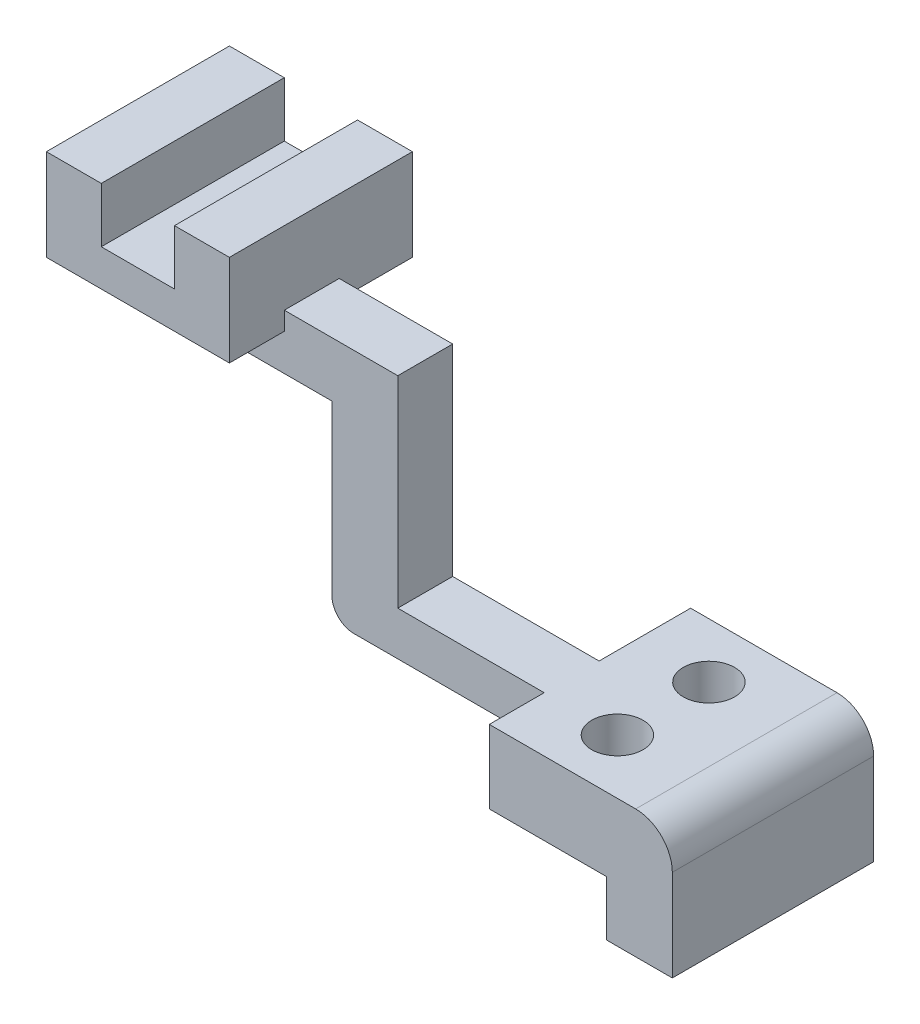
ISO-10303-21;
HEADER;
FILE_DESCRIPTION(('STEP AP214'),'2;1');
FILE_NAME('part.step','',(''),(''),'','','');
FILE_SCHEMA(('AUTOMOTIVE_DESIGN { 1 0 10303 214 1 1 1 1 }'));
ENDSEC;
DATA;
#1=APPLICATION_CONTEXT('core data for automotive mechanical design processes');
#2=APPLICATION_PROTOCOL_DEFINITION('international standard','automotive_design',2000,#1);
#3=PRODUCT_CONTEXT('',#1,'mechanical');
#4=PRODUCT('Part','Part','',(#3));
#5=PRODUCT_RELATED_PRODUCT_CATEGORY('part','',(#4));
#6=PRODUCT_DEFINITION_FORMATION('','',#4);
#7=PRODUCT_DEFINITION_CONTEXT('part definition',#1,'design');
#8=PRODUCT_DEFINITION('design','',#6,#7);
#9=PRODUCT_DEFINITION_SHAPE('','',#8);
#10=(LENGTH_UNIT() NAMED_UNIT(*) SI_UNIT(.MILLI.,.METRE.));
#11=(NAMED_UNIT(*) PLANE_ANGLE_UNIT() SI_UNIT($,.RADIAN.));
#12=(NAMED_UNIT(*) SI_UNIT($,.STERADIAN.) SOLID_ANGLE_UNIT());
#13=UNCERTAINTY_MEASURE_WITH_UNIT(LENGTH_MEASURE(1.E-05),#10,'distance_accuracy_value','');
#14=(GEOMETRIC_REPRESENTATION_CONTEXT(3) GLOBAL_UNCERTAINTY_ASSIGNED_CONTEXT((#13)) GLOBAL_UNIT_ASSIGNED_CONTEXT((#10,
#11,#12)) REPRESENTATION_CONTEXT('',''));
#15=CARTESIAN_POINT('',(0.,0.,0.));
#16=DIRECTION('',(0.,0.,1.));
#17=DIRECTION('',(1.,0.,0.));
#18=AXIS2_PLACEMENT_3D('',#15,#16,#17);
#19=CARTESIAN_POINT('',(-40.,0.,40.));
#20=DIRECTION('',(0.,0.,-1.));
#21=DIRECTION('',(-1.,0.,0.));
#22=AXIS2_PLACEMENT_3D('',#19,#20,#21);
#23=PLANE('',#22);
#24=DIRECTION('',(1.,0.,0.));
#25=VECTOR('',#24,1.);
#26=CARTESIAN_POINT('',(-121.,50.,40.));
#27=LINE('',#26,#25);
#28=CARTESIAN_POINT('',(-121.,50.,40.));
#29=VERTEX_POINT('',#28);
#30=CARTESIAN_POINT('',(-71.,50.,40.));
#31=VERTEX_POINT('',#30);
#32=EDGE_CURVE('E67',#29,#31,#27,.T.);
#33=ORIENTED_EDGE('',*,*,#32,.F.);
#34=DIRECTION('',(0.,-1.,0.));
#35=VECTOR('',#34,1.);
#36=CARTESIAN_POINT('',(-121.,40.,40.));
#37=LINE('',#36,#35);
#38=CARTESIAN_POINT('',(-121.,40.,40.));
#39=VERTEX_POINT('',#38);
#40=EDGE_CURVE('E332',#29,#39,#37,.T.);
#41=ORIENTED_EDGE('',*,*,#40,.T.);
#42=DIRECTION('',(1.,0.,0.));
#43=VECTOR('',#42,1.);
#44=CARTESIAN_POINT('',(-58.,40.,40.));
#45=LINE('',#44,#43);
#46=CARTESIAN_POINT('',(-58.,40.,40.));
#47=VERTEX_POINT('',#46);
#48=EDGE_CURVE('E333',#39,#47,#45,.T.);
#49=ORIENTED_EDGE('',*,*,#48,.T.);
#50=DIRECTION('',(0.,-1.,0.));
#51=VECTOR('',#50,1.);
#52=CARTESIAN_POINT('',(-58.,-6.00000000000004,40.));
#53=LINE('',#52,#51);
#54=CARTESIAN_POINT('',(-58.,-6.00000000000004,40.));
#55=VERTEX_POINT('',#54);
#56=EDGE_CURVE('E340',#47,#55,#53,.T.);
#57=ORIENTED_EDGE('',*,*,#56,.T.);
#58=CARTESIAN_POINT('',(-52.,-6.,40.));
#59=DIRECTION('',(0.,0.,1.));
#60=DIRECTION('',(1.,0.,0.));
#61=AXIS2_PLACEMENT_3D('',#58,#59,#60);
#62=CIRCLE('',#61,6.);
#63=CARTESIAN_POINT('',(-52.,-12.,40.));
#64=VERTEX_POINT('',#63);
#65=EDGE_CURVE('E308',#55,#64,#62,.T.);
#66=ORIENTED_EDGE('',*,*,#65,.T.);
#67=DIRECTION('',(1.,0.,0.));
#68=VECTOR('',#67,1.);
#69=CARTESIAN_POINT('',(-40.,-12.,40.));
#70=LINE('',#69,#68);
#71=CARTESIAN_POINT('',(0.,-12.,40.));
#72=VERTEX_POINT('',#71);
#73=EDGE_CURVE('E373',#64,#72,#70,.T.);
#74=ORIENTED_EDGE('',*,*,#73,.T.);
#75=DIRECTION('',(0.,1.,0.));
#76=VECTOR('',#75,1.);
#77=CARTESIAN_POINT('',(0.,0.,40.));
#78=LINE('',#77,#76);
#79=CARTESIAN_POINT('',(0.,0.,40.));
#80=VERTEX_POINT('',#79);
#81=EDGE_CURVE('E359',#72,#80,#78,.T.);
#82=ORIENTED_EDGE('',*,*,#81,.T.);
#83=DIRECTION('',(1.,0.,0.));
#84=VECTOR('',#83,1.);
#85=CARTESIAN_POINT('',(-40.,0.,40.));
#86=LINE('',#85,#84);
#87=CARTESIAN_POINT('',(-40.,0.,40.));
#88=VERTEX_POINT('',#87);
#89=EDGE_CURVE('E369',#88,#80,#86,.T.);
#90=ORIENTED_EDGE('',*,*,#89,.F.);
#91=DIRECTION('',(0.,1.,0.));
#92=VECTOR('',#91,1.);
#93=CARTESIAN_POINT('',(-40.,55.,40.));
#94=LINE('',#93,#92);
#95=CARTESIAN_POINT('',(-40.,55.,40.));
#96=VERTEX_POINT('',#95);
#97=EDGE_CURVE('E229',#88,#96,#94,.T.);
#98=ORIENTED_EDGE('',*,*,#97,.T.);
#99=DIRECTION('',(-1.,0.,0.));
#100=VECTOR('',#99,1.);
#101=CARTESIAN_POINT('',(-71.,55.,40.));
#102=LINE('',#101,#100);
#103=CARTESIAN_POINT('',(-71.,55.,40.));
#104=VERTEX_POINT('',#103);
#105=EDGE_CURVE('E329',#96,#104,#102,.T.);
#106=ORIENTED_EDGE('',*,*,#105,.T.);
#107=DIRECTION('',(0.,1.,0.));
#108=VECTOR('',#107,1.);
#109=CARTESIAN_POINT('',(-71.,50.,40.));
#110=LINE('',#109,#108);
#111=EDGE_CURVE('E61',#31,#104,#110,.T.);
#112=ORIENTED_EDGE('',*,*,#111,.F.);
#113=EDGE_LOOP('',(#33,#41,#49,#57,#66,#74,#82,#90,#98,#106,#112));
#114=FACE_BOUND('',#113,.T.);
#115=ADVANCED_FACE('F50',(#114),#23,.F.);
#116=CARTESIAN_POINT('',(0.,0.,55.));
#117=DIRECTION('',(1.,0.,0.));
#118=DIRECTION('',(0.,1.,0.));
#119=AXIS2_PLACEMENT_3D('',#116,#117,#118);
#120=PLANE('',#119);
#121=DIRECTION('',(0.,-1.,0.));
#122=VECTOR('',#121,1.);
#123=CARTESIAN_POINT('',(0.,0.,25.));
#124=LINE('',#123,#122);
#125=CARTESIAN_POINT('',(0.,0.,25.));
#126=VERTEX_POINT('',#125);
#127=CARTESIAN_POINT('',(0.,-12.,25.));
#128=VERTEX_POINT('',#127);
#129=EDGE_CURVE('E343',#126,#128,#124,.T.);
#130=ORIENTED_EDGE('',*,*,#129,.F.);
#131=DIRECTION('',(0.,0.,-1.));
#132=VECTOR('',#131,1.);
#133=CARTESIAN_POINT('',(0.,0.,55.));
#134=LINE('',#133,#132);
#135=CARTESIAN_POINT('',(0.,0.,0.));
#136=VERTEX_POINT('',#135);
#137=EDGE_CURVE('E433',#126,#136,#134,.T.);
#138=ORIENTED_EDGE('',*,*,#137,.T.);
#139=DIRECTION('',(0.,-1.,0.));
#140=VECTOR('',#139,1.);
#141=CARTESIAN_POINT('',(0.,0.,0.));
#142=LINE('',#141,#140);
#143=CARTESIAN_POINT('',(0.,-20.,0.));
#144=VERTEX_POINT('',#143);
#145=EDGE_CURVE('E414',#136,#144,#142,.T.);
#146=ORIENTED_EDGE('',*,*,#145,.T.);
#147=DIRECTION('',(0.,0.,-1.));
#148=VECTOR('',#147,1.);
#149=CARTESIAN_POINT('',(0.,-20.,55.));
#150=LINE('',#149,#148);
#151=CARTESIAN_POINT('',(0.,-20.,55.));
#152=VERTEX_POINT('',#151);
#153=EDGE_CURVE('E427',#152,#144,#150,.T.);
#154=ORIENTED_EDGE('',*,*,#153,.F.);
#155=DIRECTION('',(0.,-1.,0.));
#156=VECTOR('',#155,1.);
#157=CARTESIAN_POINT('',(0.,0.,55.));
#158=LINE('',#157,#156);
#159=CARTESIAN_POINT('',(0.,0.,55.));
#160=VERTEX_POINT('',#159);
#161=EDGE_CURVE('E394',#160,#152,#158,.T.);
#162=ORIENTED_EDGE('',*,*,#161,.F.);
#163=EDGE_CURVE('E432',#160,#80,#134,.T.);
#164=ORIENTED_EDGE('',*,*,#163,.T.);
#165=ORIENTED_EDGE('',*,*,#81,.F.);
#166=DIRECTION('',(0.,0.,1.));
#167=VECTOR('',#166,1.);
#168=CARTESIAN_POINT('',(0.,-12.,25.));
#169=LINE('',#168,#167);
#170=EDGE_CURVE('E361',#128,#72,#169,.T.);
#171=ORIENTED_EDGE('',*,*,#170,.F.);
#172=EDGE_LOOP('',(#130,#138,#146,#154,#162,#164,#165,#171));
#173=FACE_BOUND('',#172,.T.);
#174=ADVANCED_FACE('F462',(#173),#120,.F.);
#175=CARTESIAN_POINT('',(50.,0.,55.));
#176=DIRECTION('',(1.,0.,0.));
#177=DIRECTION('',(0.,0.,-1.));
#178=AXIS2_PLACEMENT_3D('',#175,#176,#177);
#179=PLANE('',#178);
#180=DIRECTION('',(0.,-1.,0.));
#181=VECTOR('',#180,1.);
#182=CARTESIAN_POINT('',(50.,0.,0.));
#183=LINE('',#182,#181);
#184=CARTESIAN_POINT('',(50.,-10.,0.));
#185=VERTEX_POINT('',#184);
#186=CARTESIAN_POINT('',(50.,-35.,0.));
#187=VERTEX_POINT('',#186);
#188=EDGE_CURVE('E407',#185,#187,#183,.T.);
#189=ORIENTED_EDGE('',*,*,#188,.F.);
#190=DIRECTION('',(0.,0.,-1.));
#191=VECTOR('',#190,1.);
#192=CARTESIAN_POINT('',(50.,-10.,55.));
#193=LINE('',#192,#191);
#194=CARTESIAN_POINT('',(50.,-10.,55.));
#195=VERTEX_POINT('',#194);
#196=EDGE_CURVE('E11',#195,#185,#193,.T.);
#197=ORIENTED_EDGE('',*,*,#196,.F.);
#198=DIRECTION('',(0.,-1.,0.));
#199=VECTOR('',#198,1.);
#200=CARTESIAN_POINT('',(50.,0.,55.));
#201=LINE('',#200,#199);
#202=CARTESIAN_POINT('',(50.,-35.,55.));
#203=VERTEX_POINT('',#202);
#204=EDGE_CURVE('E387',#195,#203,#201,.T.);
#205=ORIENTED_EDGE('',*,*,#204,.T.);
#206=DIRECTION('',(0.,0.,-1.));
#207=VECTOR('',#206,1.);
#208=CARTESIAN_POINT('',(50.,-35.,55.));
#209=LINE('',#208,#207);
#210=EDGE_CURVE('E403',#203,#187,#209,.T.);
#211=ORIENTED_EDGE('',*,*,#210,.T.);
#212=EDGE_LOOP('',(#189,#197,#205,#211));
#213=FACE_BOUND('',#212,.T.);
#214=ADVANCED_FACE('F47',(#213),#179,.T.);
#215=CARTESIAN_POINT('',(40.,-10.,55.));
#216=DIRECTION('',(0.,0.,-1.));
#217=DIRECTION('',(-1.,0.,0.));
#218=AXIS2_PLACEMENT_3D('',#215,#216,#217);
#219=CYLINDRICAL_SURFACE('',#218,10.);
#220=CARTESIAN_POINT('',(40.,-10.,0.));
#221=DIRECTION('',(0.,0.,1.));
#222=DIRECTION('',(1.,0.,0.));
#223=AXIS2_PLACEMENT_3D('',#220,#221,#222);
#224=CIRCLE('',#223,10.);
#225=CARTESIAN_POINT('',(40.,0.,0.));
#226=VERTEX_POINT('',#225);
#227=EDGE_CURVE('E406',#185,#226,#224,.T.);
#228=ORIENTED_EDGE('',*,*,#227,.T.);
#229=DIRECTION('',(0.,0.,-1.));
#230=VECTOR('',#229,1.);
#231=CARTESIAN_POINT('',(40.,0.,55.));
#232=LINE('',#231,#230);
#233=CARTESIAN_POINT('',(40.,0.,55.));
#234=VERTEX_POINT('',#233);
#235=EDGE_CURVE('E57',#234,#226,#232,.T.);
#236=ORIENTED_EDGE('',*,*,#235,.F.);
#237=CARTESIAN_POINT('',(40.,-10.,55.));
#238=DIRECTION('',(0.,0.,1.));
#239=DIRECTION('',(1.,0.,0.));
#240=AXIS2_PLACEMENT_3D('',#237,#238,#239);
#241=CIRCLE('',#240,10.);
#242=EDGE_CURVE('E386',#195,#234,#241,.T.);
#243=ORIENTED_EDGE('',*,*,#242,.F.);
#244=ORIENTED_EDGE('',*,*,#196,.T.);
#245=EDGE_LOOP('',(#228,#236,#243,#244));
#246=FACE_BOUND('',#245,.T.);
#247=ADVANCED_FACE('F827',(#246),#219,.T.);
#248=CARTESIAN_POINT('',(0.,0.,55.));
#249=DIRECTION('',(0.,1.,0.));
#250=DIRECTION('',(0.,0.,1.));
#251=AXIS2_PLACEMENT_3D('',#248,#249,#250);
#252=PLANE('',#251);
#253=ORIENTED_EDGE('',*,*,#137,.F.);
#254=DIRECTION('',(1.,0.,0.));
#255=VECTOR('',#254,1.);
#256=CARTESIAN_POINT('',(-40.,0.,25.));
#257=LINE('',#256,#255);
#258=CARTESIAN_POINT('',(-40.,0.,25.));
#259=VERTEX_POINT('',#258);
#260=EDGE_CURVE('E360',#259,#126,#257,.T.);
#261=ORIENTED_EDGE('',*,*,#260,.F.);
#262=DIRECTION('',(0.,0.,-1.));
#263=VECTOR('',#262,1.);
#264=CARTESIAN_POINT('',(-40.,0.,25.));
#265=LINE('',#264,#263);
#266=EDGE_CURVE('E358',#88,#259,#265,.T.);
#267=ORIENTED_EDGE('',*,*,#266,.F.);
#268=ORIENTED_EDGE('',*,*,#89,.T.);
#269=ORIENTED_EDGE('',*,*,#163,.F.);
#270=DIRECTION('',(1.,0.,0.));
#271=VECTOR('',#270,1.);
#272=CARTESIAN_POINT('',(0.,0.,55.));
#273=LINE('',#272,#271);
#274=EDGE_CURVE('E395',#160,#234,#273,.T.);
#275=ORIENTED_EDGE('',*,*,#274,.T.);
#276=ORIENTED_EDGE('',*,*,#235,.T.);
#277=DIRECTION('',(1.,0.,0.));
#278=VECTOR('',#277,1.);
#279=CARTESIAN_POINT('',(0.,0.,0.));
#280=LINE('',#279,#278);
#281=EDGE_CURVE('E415',#136,#226,#280,.T.);
#282=ORIENTED_EDGE('',*,*,#281,.F.);
#283=EDGE_LOOP('',(#253,#261,#267,#268,#269,#275,#276,#282));
#284=FACE_BOUND('',#283,.T.);
#285=CARTESIAN_POINT('',(20.,0.,15.));
#286=DIRECTION('',(0.,1.,0.));
#287=DIRECTION('',(0.,0.,1.));
#288=AXIS2_PLACEMENT_3D('',#285,#286,#287);
#289=CIRCLE('',#288,7.);
#290=CARTESIAN_POINT('',(20.,0.,22.));
#291=VERTEX_POINT('',#290);
#292=EDGE_CURVE('E379',#291,#291,#289,.T.);
#293=ORIENTED_EDGE('',*,*,#292,.F.);
#294=EDGE_LOOP('',(#293));
#295=FACE_BOUND('',#294,.T.);
#296=CARTESIAN_POINT('',(20.,0.,40.));
#297=DIRECTION('',(0.,1.,0.));
#298=DIRECTION('',(0.,0.,1.));
#299=AXIS2_PLACEMENT_3D('',#296,#297,#298);
#300=CIRCLE('',#299,7.);
#301=CARTESIAN_POINT('',(20.,0.,47.));
#302=VERTEX_POINT('',#301);
#303=EDGE_CURVE('E378',#302,#302,#300,.T.);
#304=ORIENTED_EDGE('',*,*,#303,.F.);
#305=EDGE_LOOP('',(#304));
#306=FACE_BOUND('',#305,.T.);
#307=ADVANCED_FACE('F516',(#284,#295,#306),#252,.T.);
#308=CARTESIAN_POINT('',(0.,-20.,55.));
#309=DIRECTION('',(0.,1.,0.));
#310=DIRECTION('',(0.,0.,1.));
#311=AXIS2_PLACEMENT_3D('',#308,#309,#310);
#312=PLANE('',#311);
#313=CARTESIAN_POINT('',(20.,-20.,15.));
#314=DIRECTION('',(0.,1.,0.));
#315=DIRECTION('',(0.,0.,1.));
#316=AXIS2_PLACEMENT_3D('',#313,#314,#315);
#317=CIRCLE('',#316,7.);
#318=CARTESIAN_POINT('',(20.,-20.,22.));
#319=VERTEX_POINT('',#318);
#320=EDGE_CURVE('E51',#319,#319,#317,.T.);
#321=ORIENTED_EDGE('',*,*,#320,.T.);
#322=EDGE_LOOP('',(#321));
#323=FACE_BOUND('',#322,.T.);
#324=CARTESIAN_POINT('',(20.,-20.,40.));
#325=DIRECTION('',(0.,1.,0.));
#326=DIRECTION('',(0.,0.,1.));
#327=AXIS2_PLACEMENT_3D('',#324,#325,#326);
#328=CIRCLE('',#327,7.);
#329=CARTESIAN_POINT('',(20.,-20.,47.));
#330=VERTEX_POINT('',#329);
#331=EDGE_CURVE('E384',#330,#330,#328,.T.);
#332=ORIENTED_EDGE('',*,*,#331,.T.);
#333=EDGE_LOOP('',(#332));
#334=FACE_BOUND('',#333,.T.);
#335=DIRECTION('',(1.,0.,0.));
#336=VECTOR('',#335,1.);
#337=CARTESIAN_POINT('',(0.,-20.,0.));
#338=LINE('',#337,#336);
#339=CARTESIAN_POINT('',(32.,-20.,0.));
#340=VERTEX_POINT('',#339);
#341=EDGE_CURVE('E417',#144,#340,#338,.T.);
#342=ORIENTED_EDGE('',*,*,#341,.T.);
#343=DIRECTION('',(0.,0.,-1.));
#344=VECTOR('',#343,1.);
#345=CARTESIAN_POINT('',(32.,-20.,55.));
#346=LINE('',#345,#344);
#347=CARTESIAN_POINT('',(32.,-20.,55.));
#348=VERTEX_POINT('',#347);
#349=EDGE_CURVE('E426',#348,#340,#346,.T.);
#350=ORIENTED_EDGE('',*,*,#349,.F.);
#351=DIRECTION('',(1.,0.,0.));
#352=VECTOR('',#351,1.);
#353=CARTESIAN_POINT('',(0.,-20.,55.));
#354=LINE('',#353,#352);
#355=EDGE_CURVE('E397',#152,#348,#354,.T.);
#356=ORIENTED_EDGE('',*,*,#355,.F.);
#357=ORIENTED_EDGE('',*,*,#153,.T.);
#358=EDGE_LOOP('',(#342,#350,#356,#357));
#359=FACE_BOUND('',#358,.T.);
#360=ADVANCED_FACE('F445',(#323,#334,#359),#312,.F.);
#361=CARTESIAN_POINT('',(32.,0.,55.));
#362=DIRECTION('',(-1.,0.,0.));
#363=DIRECTION('',(0.,0.,1.));
#364=AXIS2_PLACEMENT_3D('',#361,#362,#363);
#365=PLANE('',#364);
#366=DIRECTION('',(0.,1.,0.));
#367=VECTOR('',#366,1.);
#368=CARTESIAN_POINT('',(32.,0.,0.));
#369=LINE('',#368,#367);
#370=CARTESIAN_POINT('',(32.,-35.,0.));
#371=VERTEX_POINT('',#370);
#372=EDGE_CURVE('E420',#371,#340,#369,.T.);
#373=ORIENTED_EDGE('',*,*,#372,.F.);
#374=DIRECTION('',(0.,0.,-1.));
#375=VECTOR('',#374,1.);
#376=CARTESIAN_POINT('',(32.,-35.,55.));
#377=LINE('',#376,#375);
#378=CARTESIAN_POINT('',(32.,-35.,55.));
#379=VERTEX_POINT('',#378);
#380=EDGE_CURVE('E428',#379,#371,#377,.T.);
#381=ORIENTED_EDGE('',*,*,#380,.F.);
#382=DIRECTION('',(0.,1.,0.));
#383=VECTOR('',#382,1.);
#384=CARTESIAN_POINT('',(32.,0.,55.));
#385=LINE('',#384,#383);
#386=EDGE_CURVE('E398',#379,#348,#385,.T.);
#387=ORIENTED_EDGE('',*,*,#386,.T.);
#388=ORIENTED_EDGE('',*,*,#349,.T.);
#389=EDGE_LOOP('',(#373,#381,#387,#388));
#390=FACE_BOUND('',#389,.T.);
#391=ADVANCED_FACE('F804',(#390),#365,.T.);
#392=CARTESIAN_POINT('',(0.,-35.,55.));
#393=DIRECTION('',(0.,-1.,0.));
#394=DIRECTION('',(0.,0.,-1.));
#395=AXIS2_PLACEMENT_3D('',#392,#393,#394);
#396=PLANE('',#395);
#397=DIRECTION('',(-1.,0.,0.));
#398=VECTOR('',#397,1.);
#399=CARTESIAN_POINT('',(0.,-35.,0.));
#400=LINE('',#399,#398);
#401=EDGE_CURVE('E388',#187,#371,#400,.T.);
#402=ORIENTED_EDGE('',*,*,#401,.F.);
#403=ORIENTED_EDGE('',*,*,#210,.F.);
#404=DIRECTION('',(-1.,0.,0.));
#405=VECTOR('',#404,1.);
#406=CARTESIAN_POINT('',(0.,-35.,55.));
#407=LINE('',#406,#405);
#408=EDGE_CURVE('E405',#203,#379,#407,.T.);
#409=ORIENTED_EDGE('',*,*,#408,.T.);
#410=ORIENTED_EDGE('',*,*,#380,.T.);
#411=EDGE_LOOP('',(#402,#403,#409,#410));
#412=FACE_BOUND('',#411,.T.);
#413=ADVANCED_FACE('F800',(#412),#396,.T.);
#414=CARTESIAN_POINT('',(0.,0.,55.));
#415=DIRECTION('',(0.,0.,1.));
#416=DIRECTION('',(1.,0.,0.));
#417=AXIS2_PLACEMENT_3D('',#414,#415,#416);
#418=PLANE('',#417);
#419=ORIENTED_EDGE('',*,*,#204,.F.);
#420=ORIENTED_EDGE('',*,*,#242,.T.);
#421=ORIENTED_EDGE('',*,*,#274,.F.);
#422=ORIENTED_EDGE('',*,*,#161,.T.);
#423=ORIENTED_EDGE('',*,*,#355,.T.);
#424=ORIENTED_EDGE('',*,*,#386,.F.);
#425=ORIENTED_EDGE('',*,*,#408,.F.);
#426=EDGE_LOOP('',(#419,#420,#421,#422,#423,#424,#425));
#427=FACE_BOUND('',#426,.T.);
#428=ADVANCED_FACE('F533',(#427),#418,.T.);
#429=CARTESIAN_POINT('',(0.,0.,0.));
#430=DIRECTION('',(0.,0.,1.));
#431=DIRECTION('',(1.,0.,0.));
#432=AXIS2_PLACEMENT_3D('',#429,#430,#431);
#433=PLANE('',#432);
#434=ORIENTED_EDGE('',*,*,#188,.T.);
#435=ORIENTED_EDGE('',*,*,#401,.T.);
#436=ORIENTED_EDGE('',*,*,#372,.T.);
#437=ORIENTED_EDGE('',*,*,#341,.F.);
#438=ORIENTED_EDGE('',*,*,#145,.F.);
#439=ORIENTED_EDGE('',*,*,#281,.T.);
#440=ORIENTED_EDGE('',*,*,#227,.F.);
#441=EDGE_LOOP('',(#434,#435,#436,#437,#438,#439,#440));
#442=FACE_BOUND('',#441,.T.);
#443=ADVANCED_FACE('F457',(#442),#433,.F.);
#444=CARTESIAN_POINT('',(20.,-22.,40.));
#445=DIRECTION('',(0.,1.,0.));
#446=DIRECTION('',(0.,0.,1.));
#447=AXIS2_PLACEMENT_3D('',#444,#445,#446);
#448=CYLINDRICAL_SURFACE('',#447,7.);
#449=ORIENTED_EDGE('',*,*,#303,.T.);
#450=EDGE_LOOP('',(#449));
#451=FACE_BOUND('',#450,.T.);
#452=ORIENTED_EDGE('',*,*,#331,.F.);
#453=EDGE_LOOP('',(#452));
#454=FACE_BOUND('',#453,.T.);
#455=ADVANCED_FACE('F450',(#451,#454),#448,.F.);
#456=CARTESIAN_POINT('',(20.,-22.,15.));
#457=DIRECTION('',(0.,1.,0.));
#458=DIRECTION('',(0.,0.,1.));
#459=AXIS2_PLACEMENT_3D('',#456,#457,#458);
#460=CYLINDRICAL_SURFACE('',#459,7.);
#461=ORIENTED_EDGE('',*,*,#292,.T.);
#462=EDGE_LOOP('',(#461));
#463=FACE_BOUND('',#462,.T.);
#464=ORIENTED_EDGE('',*,*,#320,.F.);
#465=EDGE_LOOP('',(#464));
#466=FACE_BOUND('',#465,.T.);
#467=ADVANCED_FACE('F443',(#463,#466),#460,.F.);
#468=CARTESIAN_POINT('',(-40.,0.,25.));
#469=DIRECTION('',(0.,0.,1.));
#470=DIRECTION('',(1.,0.,0.));
#471=AXIS2_PLACEMENT_3D('',#468,#469,#470);
#472=PLANE('',#471);
#473=ORIENTED_EDGE('',*,*,#129,.T.);
#474=DIRECTION('',(1.,0.,0.));
#475=VECTOR('',#474,1.);
#476=CARTESIAN_POINT('',(-40.,-12.,25.));
#477=LINE('',#476,#475);
#478=CARTESIAN_POINT('',(-52.,-12.,25.));
#479=VERTEX_POINT('',#478);
#480=EDGE_CURVE('E376',#479,#128,#477,.T.);
#481=ORIENTED_EDGE('',*,*,#480,.F.);
#482=CARTESIAN_POINT('',(-52.,-6.,25.));
#483=DIRECTION('',(0.,0.,1.));
#484=DIRECTION('',(1.,0.,0.));
#485=AXIS2_PLACEMENT_3D('',#482,#483,#484);
#486=CIRCLE('',#485,6.);
#487=CARTESIAN_POINT('',(-58.,-6.00000000000004,25.));
#488=VERTEX_POINT('',#487);
#489=EDGE_CURVE('E321',#488,#479,#486,.T.);
#490=ORIENTED_EDGE('',*,*,#489,.F.);
#491=DIRECTION('',(0.,-1.,0.));
#492=VECTOR('',#491,1.);
#493=CARTESIAN_POINT('',(-58.,-6.00000000000004,25.));
#494=LINE('',#493,#492);
#495=CARTESIAN_POINT('',(-58.,40.,25.));
#496=VERTEX_POINT('',#495);
#497=EDGE_CURVE('E322',#496,#488,#494,.T.);
#498=ORIENTED_EDGE('',*,*,#497,.F.);
#499=DIRECTION('',(1.,0.,0.));
#500=VECTOR('',#499,1.);
#501=CARTESIAN_POINT('',(-58.,40.,25.));
#502=LINE('',#501,#500);
#503=CARTESIAN_POINT('',(-121.,40.,25.));
#504=VERTEX_POINT('',#503);
#505=EDGE_CURVE('E319',#504,#496,#502,.T.);
#506=ORIENTED_EDGE('',*,*,#505,.F.);
#507=DIRECTION('',(0.,-1.,0.));
#508=VECTOR('',#507,1.);
#509=CARTESIAN_POINT('',(-121.,40.,25.));
#510=LINE('',#509,#508);
#511=CARTESIAN_POINT('',(-121.,50.,25.));
#512=VERTEX_POINT('',#511);
#513=EDGE_CURVE('E314',#512,#504,#510,.T.);
#514=ORIENTED_EDGE('',*,*,#513,.F.);
#515=DIRECTION('',(-1.,0.,0.));
#516=VECTOR('',#515,1.);
#517=CARTESIAN_POINT('',(-121.,50.,25.));
#518=LINE('',#517,#516);
#519=CARTESIAN_POINT('',(-71.,50.,25.));
#520=VERTEX_POINT('',#519);
#521=EDGE_CURVE('E312',#520,#512,#518,.T.);
#522=ORIENTED_EDGE('',*,*,#521,.F.);
#523=DIRECTION('',(0.,-1.,0.));
#524=VECTOR('',#523,1.);
#525=CARTESIAN_POINT('',(-71.,50.,25.));
#526=LINE('',#525,#524);
#527=CARTESIAN_POINT('',(-71.,55.,25.));
#528=VERTEX_POINT('',#527);
#529=EDGE_CURVE('E311',#528,#520,#526,.T.);
#530=ORIENTED_EDGE('',*,*,#529,.F.);
#531=DIRECTION('',(-1.,0.,0.));
#532=VECTOR('',#531,1.);
#533=CARTESIAN_POINT('',(-71.,55.,25.));
#534=LINE('',#533,#532);
#535=CARTESIAN_POINT('',(-40.,55.,25.));
#536=VERTEX_POINT('',#535);
#537=EDGE_CURVE('E310',#536,#528,#534,.T.);
#538=ORIENTED_EDGE('',*,*,#537,.F.);
#539=DIRECTION('',(0.,1.,0.));
#540=VECTOR('',#539,1.);
#541=CARTESIAN_POINT('',(-40.,55.,25.));
#542=LINE('',#541,#540);
#543=EDGE_CURVE('E302',#259,#536,#542,.T.);
#544=ORIENTED_EDGE('',*,*,#543,.F.);
#545=ORIENTED_EDGE('',*,*,#260,.T.);
#546=EDGE_LOOP('',(#473,#481,#490,#498,#506,#514,#522,#530,#538,#544,#545));
#547=FACE_BOUND('',#546,.T.);
#548=ADVANCED_FACE('F447',(#547),#472,.F.);
#549=CARTESIAN_POINT('',(-40.,-12.,25.));
#550=DIRECTION('',(0.,1.,0.));
#551=DIRECTION('',(-1.,0.,0.));
#552=AXIS2_PLACEMENT_3D('',#549,#550,#551);
#553=PLANE('',#552);
#554=ORIENTED_EDGE('',*,*,#170,.T.);
#555=ORIENTED_EDGE('',*,*,#73,.F.);
#556=DIRECTION('',(0.,0.,1.));
#557=VECTOR('',#556,1.);
#558=CARTESIAN_POINT('',(-52.,-12.,25.));
#559=LINE('',#558,#557);
#560=EDGE_CURVE('E345',#479,#64,#559,.T.);
#561=ORIENTED_EDGE('',*,*,#560,.F.);
#562=ORIENTED_EDGE('',*,*,#480,.T.);
#563=EDGE_LOOP('',(#554,#555,#561,#562));
#564=FACE_BOUND('',#563,.T.);
#565=ADVANCED_FACE('F453',(#564),#553,.F.);
#566=CARTESIAN_POINT('',(-52.,-6.,25.));
#567=DIRECTION('',(0.,0.,1.));
#568=DIRECTION('',(1.,0.,0.));
#569=AXIS2_PLACEMENT_3D('',#566,#567,#568);
#570=CYLINDRICAL_SURFACE('',#569,6.);
#571=ORIENTED_EDGE('',*,*,#65,.F.);
#572=DIRECTION('',(0.,0.,1.));
#573=VECTOR('',#572,1.);
#574=CARTESIAN_POINT('',(-58.,-6.00000000000004,25.));
#575=LINE('',#574,#573);
#576=EDGE_CURVE('E346',#488,#55,#575,.T.);
#577=ORIENTED_EDGE('',*,*,#576,.F.);
#578=ORIENTED_EDGE('',*,*,#489,.T.);
#579=ORIENTED_EDGE('',*,*,#560,.T.);
#580=EDGE_LOOP('',(#571,#577,#578,#579));
#581=FACE_BOUND('',#580,.T.);
#582=ADVANCED_FACE('F476',(#581),#570,.T.);
#583=CARTESIAN_POINT('',(-58.,-6.00000000000004,25.));
#584=DIRECTION('',(-1.,0.,0.));
#585=DIRECTION('',(0.,0.,1.));
#586=AXIS2_PLACEMENT_3D('',#583,#584,#585);
#587=PLANE('',#586);
#588=ORIENTED_EDGE('',*,*,#56,.F.);
#589=DIRECTION('',(0.,0.,1.));
#590=VECTOR('',#589,1.);
#591=CARTESIAN_POINT('',(-58.,40.,25.));
#592=LINE('',#591,#590);
#593=EDGE_CURVE('E347',#496,#47,#592,.T.);
#594=ORIENTED_EDGE('',*,*,#593,.F.);
#595=ORIENTED_EDGE('',*,*,#497,.T.);
#596=ORIENTED_EDGE('',*,*,#576,.T.);
#597=EDGE_LOOP('',(#588,#594,#595,#596));
#598=FACE_BOUND('',#597,.T.);
#599=ADVANCED_FACE('F482',(#598),#587,.T.);
#600=CARTESIAN_POINT('',(-58.,40.,25.));
#601=DIRECTION('',(0.,-1.,0.));
#602=DIRECTION('',(0.,0.,-1.));
#603=AXIS2_PLACEMENT_3D('',#600,#601,#602);
#604=PLANE('',#603);
#605=ORIENTED_EDGE('',*,*,#48,.F.);
#606=DIRECTION('',(0.,0.,1.));
#607=VECTOR('',#606,1.);
#608=CARTESIAN_POINT('',(-121.,40.,25.));
#609=LINE('',#608,#607);
#610=EDGE_CURVE('E349',#504,#39,#609,.T.);
#611=ORIENTED_EDGE('',*,*,#610,.F.);
#612=ORIENTED_EDGE('',*,*,#505,.T.);
#613=ORIENTED_EDGE('',*,*,#593,.T.);
#614=EDGE_LOOP('',(#605,#611,#612,#613));
#615=FACE_BOUND('',#614,.T.);
#616=ADVANCED_FACE('F492',(#615),#604,.T.);
#617=CARTESIAN_POINT('',(-121.,40.,25.));
#618=DIRECTION('',(-1.,0.,0.));
#619=DIRECTION('',(0.,0.,1.));
#620=AXIS2_PLACEMENT_3D('',#617,#618,#619);
#621=PLANE('',#620);
#622=ORIENTED_EDGE('',*,*,#40,.F.);
#623=DIRECTION('',(0.,0.,-1.));
#624=VECTOR('',#623,1.);
#625=CARTESIAN_POINT('',(-121.,50.,55.));
#626=LINE('',#625,#624);
#627=CARTESIAN_POINT('',(-121.,50.,55.));
#628=VERTEX_POINT('',#627);
#629=EDGE_CURVE('E240',#628,#29,#626,.T.);
#630=ORIENTED_EDGE('',*,*,#629,.F.);
#631=DIRECTION('',(0.,-1.,0.));
#632=VECTOR('',#631,1.);
#633=CARTESIAN_POINT('',(-121.,75.,55.));
#634=LINE('',#633,#632);
#635=CARTESIAN_POINT('',(-121.,75.,55.));
#636=VERTEX_POINT('',#635);
#637=EDGE_CURVE('E234',#636,#628,#634,.T.);
#638=ORIENTED_EDGE('',*,*,#637,.F.);
#639=DIRECTION('',(0.,0.,1.));
#640=VECTOR('',#639,1.);
#641=CARTESIAN_POINT('',(-121.,75.,5.));
#642=LINE('',#641,#640);
#643=CARTESIAN_POINT('',(-121.,75.,5.));
#644=VERTEX_POINT('',#643);
#645=EDGE_CURVE('E219',#644,#636,#642,.T.);
#646=ORIENTED_EDGE('',*,*,#645,.F.);
#647=DIRECTION('',(0.,-1.,0.));
#648=VECTOR('',#647,1.);
#649=CARTESIAN_POINT('',(-121.,75.,5.));
#650=LINE('',#649,#648);
#651=CARTESIAN_POINT('',(-121.,50.,5.));
#652=VERTEX_POINT('',#651);
#653=EDGE_CURVE('E269',#644,#652,#650,.T.);
#654=ORIENTED_EDGE('',*,*,#653,.T.);
#655=DIRECTION('',(0.,0.,1.));
#656=VECTOR('',#655,1.);
#657=CARTESIAN_POINT('',(-121.,50.,5.));
#658=LINE('',#657,#656);
#659=EDGE_CURVE('E289',#652,#512,#658,.T.);
#660=ORIENTED_EDGE('',*,*,#659,.T.);
#661=ORIENTED_EDGE('',*,*,#513,.T.);
#662=ORIENTED_EDGE('',*,*,#610,.T.);
#663=EDGE_LOOP('',(#622,#630,#638,#646,#654,#660,#661,#662));
#664=FACE_BOUND('',#663,.T.);
#665=ADVANCED_FACE('F232',(#664),#621,.T.);
#666=CARTESIAN_POINT('',(-71.,55.,25.));
#667=DIRECTION('',(0.,1.,0.));
#668=DIRECTION('',(0.,0.,1.));
#669=AXIS2_PLACEMENT_3D('',#666,#667,#668);
#670=PLANE('',#669);
#671=ORIENTED_EDGE('',*,*,#105,.F.);
#672=DIRECTION('',(0.,0.,1.));
#673=VECTOR('',#672,1.);
#674=CARTESIAN_POINT('',(-40.,55.,25.));
#675=LINE('',#674,#673);
#676=EDGE_CURVE('E330',#536,#96,#675,.T.);
#677=ORIENTED_EDGE('',*,*,#676,.F.);
#678=ORIENTED_EDGE('',*,*,#537,.T.);
#679=DIRECTION('',(0.,0.,1.));
#680=VECTOR('',#679,1.);
#681=CARTESIAN_POINT('',(-71.,55.,25.));
#682=LINE('',#681,#680);
#683=EDGE_CURVE('E354',#528,#104,#682,.T.);
#684=ORIENTED_EDGE('',*,*,#683,.T.);
#685=EDGE_LOOP('',(#671,#677,#678,#684));
#686=FACE_BOUND('',#685,.T.);
#687=ADVANCED_FACE('F511',(#686),#670,.T.);
#688=CARTESIAN_POINT('',(-40.,55.,25.));
#689=DIRECTION('',(1.,0.,0.));
#690=DIRECTION('',(0.,0.,-1.));
#691=AXIS2_PLACEMENT_3D('',#688,#689,#690);
#692=PLANE('',#691);
#693=ORIENTED_EDGE('',*,*,#97,.F.);
#694=ORIENTED_EDGE('',*,*,#266,.T.);
#695=ORIENTED_EDGE('',*,*,#543,.T.);
#696=ORIENTED_EDGE('',*,*,#676,.T.);
#697=EDGE_LOOP('',(#693,#694,#695,#696));
#698=FACE_BOUND('',#697,.T.);
#699=ADVANCED_FACE('F474',(#698),#692,.T.);
#700=CARTESIAN_POINT('',(-121.,50.,5.));
#701=DIRECTION('',(0.,-1.,0.));
#702=DIRECTION('',(0.,0.,-1.));
#703=AXIS2_PLACEMENT_3D('',#700,#701,#702);
#704=PLANE('',#703);
#705=ORIENTED_EDGE('',*,*,#521,.T.);
#706=ORIENTED_EDGE('',*,*,#659,.F.);
#707=DIRECTION('',(1.,0.,0.));
#708=VECTOR('',#707,1.);
#709=CARTESIAN_POINT('',(-121.,50.,5.));
#710=LINE('',#709,#708);
#711=CARTESIAN_POINT('',(-71.,50.,5.));
#712=VERTEX_POINT('',#711);
#713=EDGE_CURVE('E270',#652,#712,#710,.T.);
#714=ORIENTED_EDGE('',*,*,#713,.T.);
#715=DIRECTION('',(0.,0.,1.));
#716=VECTOR('',#715,1.);
#717=CARTESIAN_POINT('',(-71.,50.,5.));
#718=LINE('',#717,#716);
#719=EDGE_CURVE('E299',#712,#520,#718,.T.);
#720=ORIENTED_EDGE('',*,*,#719,.T.);
#721=EDGE_LOOP('',(#705,#706,#714,#720));
#722=FACE_BOUND('',#721,.T.);
#723=ADVANCED_FACE('F499',(#722),#704,.T.);
#724=CARTESIAN_POINT('',(-71.,50.,5.));
#725=DIRECTION('',(1.,0.,0.));
#726=DIRECTION('',(0.,0.,-1.));
#727=AXIS2_PLACEMENT_3D('',#724,#725,#726);
#728=PLANE('',#727);
#729=ORIENTED_EDGE('',*,*,#529,.T.);
#730=ORIENTED_EDGE('',*,*,#719,.F.);
#731=DIRECTION('',(0.,1.,0.));
#732=VECTOR('',#731,1.);
#733=CARTESIAN_POINT('',(-71.,50.,5.));
#734=LINE('',#733,#732);
#735=CARTESIAN_POINT('',(-71.,75.,5.));
#736=VERTEX_POINT('',#735);
#737=EDGE_CURVE('E271',#712,#736,#734,.T.);
#738=ORIENTED_EDGE('',*,*,#737,.T.);
#739=DIRECTION('',(0.,0.,1.));
#740=VECTOR('',#739,1.);
#741=CARTESIAN_POINT('',(-71.,75.,5.));
#742=LINE('',#741,#740);
#743=CARTESIAN_POINT('',(-71.,75.,55.));
#744=VERTEX_POINT('',#743);
#745=EDGE_CURVE('E300',#736,#744,#742,.T.);
#746=ORIENTED_EDGE('',*,*,#745,.T.);
#747=DIRECTION('',(0.,1.,0.));
#748=VECTOR('',#747,1.);
#749=CARTESIAN_POINT('',(-71.,50.,55.));
#750=LINE('',#749,#748);
#751=CARTESIAN_POINT('',(-71.,50.,55.));
#752=VERTEX_POINT('',#751);
#753=EDGE_CURVE('E252',#752,#744,#750,.T.);
#754=ORIENTED_EDGE('',*,*,#753,.F.);
#755=DIRECTION('',(0.,0.,-1.));
#756=VECTOR('',#755,1.);
#757=CARTESIAN_POINT('',(-71.,50.,55.));
#758=LINE('',#757,#756);
#759=EDGE_CURVE('E262',#752,#31,#758,.T.);
#760=ORIENTED_EDGE('',*,*,#759,.T.);
#761=ORIENTED_EDGE('',*,*,#111,.T.);
#762=ORIENTED_EDGE('',*,*,#683,.F.);
#763=EDGE_LOOP('',(#729,#730,#738,#746,#754,#760,#761,#762));
#764=FACE_BOUND('',#763,.T.);
#765=ADVANCED_FACE('F510',(#764),#728,.T.);
#766=CARTESIAN_POINT('',(-106.,75.,5.));
#767=DIRECTION('',(0.,1.,0.));
#768=DIRECTION('',(0.,0.,1.));
#769=AXIS2_PLACEMENT_3D('',#766,#767,#768);
#770=PLANE('',#769);
#771=ORIENTED_EDGE('',*,*,#645,.T.);
#772=DIRECTION('',(-1.,0.,0.));
#773=VECTOR('',#772,1.);
#774=CARTESIAN_POINT('',(-106.,75.,55.));
#775=LINE('',#774,#773);
#776=CARTESIAN_POINT('',(-106.,75.,55.));
#777=VERTEX_POINT('',#776);
#778=EDGE_CURVE('E223',#777,#636,#775,.T.);
#779=ORIENTED_EDGE('',*,*,#778,.F.);
#780=DIRECTION('',(0.,0.,1.));
#781=VECTOR('',#780,1.);
#782=CARTESIAN_POINT('',(-106.,75.,5.));
#783=LINE('',#782,#781);
#784=CARTESIAN_POINT('',(-106.,75.,5.));
#785=VERTEX_POINT('',#784);
#786=EDGE_CURVE('E233',#785,#777,#783,.T.);
#787=ORIENTED_EDGE('',*,*,#786,.F.);
#788=DIRECTION('',(-1.,0.,0.));
#789=VECTOR('',#788,1.);
#790=CARTESIAN_POINT('',(-106.,75.,5.));
#791=LINE('',#790,#789);
#792=EDGE_CURVE('E228',#785,#644,#791,.T.);
#793=ORIENTED_EDGE('',*,*,#792,.T.);
#794=EDGE_LOOP('',(#771,#779,#787,#793));
#795=FACE_BOUND('',#794,.T.);
#796=ADVANCED_FACE('F222',(#795),#770,.T.);
#797=CARTESIAN_POINT('',(-106.,60.,5.));
#798=DIRECTION('',(1.,0.,0.));
#799=DIRECTION('',(0.,0.,-1.));
#800=AXIS2_PLACEMENT_3D('',#797,#798,#799);
#801=PLANE('',#800);
#802=ORIENTED_EDGE('',*,*,#786,.T.);
#803=DIRECTION('',(0.,1.,0.));
#804=VECTOR('',#803,1.);
#805=CARTESIAN_POINT('',(-106.,60.,55.));
#806=LINE('',#805,#804);
#807=CARTESIAN_POINT('',(-106.,60.,55.));
#808=VERTEX_POINT('',#807);
#809=EDGE_CURVE('E246',#808,#777,#806,.T.);
#810=ORIENTED_EDGE('',*,*,#809,.F.);
#811=DIRECTION('',(0.,0.,1.));
#812=VECTOR('',#811,1.);
#813=CARTESIAN_POINT('',(-106.,60.,5.));
#814=LINE('',#813,#812);
#815=CARTESIAN_POINT('',(-106.,60.,5.));
#816=VERTEX_POINT('',#815);
#817=EDGE_CURVE('E293',#816,#808,#814,.T.);
#818=ORIENTED_EDGE('',*,*,#817,.F.);
#819=DIRECTION('',(0.,1.,0.));
#820=VECTOR('',#819,1.);
#821=CARTESIAN_POINT('',(-106.,60.,5.));
#822=LINE('',#821,#820);
#823=EDGE_CURVE('E284',#816,#785,#822,.T.);
#824=ORIENTED_EDGE('',*,*,#823,.T.);
#825=EDGE_LOOP('',(#802,#810,#818,#824));
#826=FACE_BOUND('',#825,.T.);
#827=ADVANCED_FACE('F551',(#826),#801,.T.);
#828=CARTESIAN_POINT('',(-86.,60.,5.));
#829=DIRECTION('',(0.,1.,0.));
#830=DIRECTION('',(0.,0.,1.));
#831=AXIS2_PLACEMENT_3D('',#828,#829,#830);
#832=PLANE('',#831);
#833=ORIENTED_EDGE('',*,*,#817,.T.);
#834=DIRECTION('',(-1.,0.,0.));
#835=VECTOR('',#834,1.);
#836=CARTESIAN_POINT('',(-86.,60.,55.));
#837=LINE('',#836,#835);
#838=CARTESIAN_POINT('',(-86.,60.,55.));
#839=VERTEX_POINT('',#838);
#840=EDGE_CURVE('E258',#839,#808,#837,.T.);
#841=ORIENTED_EDGE('',*,*,#840,.F.);
#842=DIRECTION('',(0.,0.,1.));
#843=VECTOR('',#842,1.);
#844=CARTESIAN_POINT('',(-86.,60.,5.));
#845=LINE('',#844,#843);
#846=CARTESIAN_POINT('',(-86.,60.,5.));
#847=VERTEX_POINT('',#846);
#848=EDGE_CURVE('E291',#847,#839,#845,.T.);
#849=ORIENTED_EDGE('',*,*,#848,.F.);
#850=DIRECTION('',(-1.,0.,0.));
#851=VECTOR('',#850,1.);
#852=CARTESIAN_POINT('',(-86.,60.,5.));
#853=LINE('',#852,#851);
#854=EDGE_CURVE('E285',#847,#816,#853,.T.);
#855=ORIENTED_EDGE('',*,*,#854,.T.);
#856=EDGE_LOOP('',(#833,#841,#849,#855));
#857=FACE_BOUND('',#856,.T.);
#858=ADVANCED_FACE('F550',(#857),#832,.T.);
#859=CARTESIAN_POINT('',(-86.,75.,5.));
#860=DIRECTION('',(-1.,0.,0.));
#861=DIRECTION('',(0.,0.,1.));
#862=AXIS2_PLACEMENT_3D('',#859,#860,#861);
#863=PLANE('',#862);
#864=ORIENTED_EDGE('',*,*,#848,.T.);
#865=DIRECTION('',(0.,-1.,0.));
#866=VECTOR('',#865,1.);
#867=CARTESIAN_POINT('',(-86.,75.,55.));
#868=LINE('',#867,#866);
#869=CARTESIAN_POINT('',(-86.,75.,55.));
#870=VERTEX_POINT('',#869);
#871=EDGE_CURVE('E260',#870,#839,#868,.T.);
#872=ORIENTED_EDGE('',*,*,#871,.F.);
#873=DIRECTION('',(0.,0.,1.));
#874=VECTOR('',#873,1.);
#875=CARTESIAN_POINT('',(-86.,75.,5.));
#876=LINE('',#875,#874);
#877=CARTESIAN_POINT('',(-86.,75.,5.));
#878=VERTEX_POINT('',#877);
#879=EDGE_CURVE('E294',#878,#870,#876,.T.);
#880=ORIENTED_EDGE('',*,*,#879,.F.);
#881=DIRECTION('',(0.,-1.,0.));
#882=VECTOR('',#881,1.);
#883=CARTESIAN_POINT('',(-86.,75.,5.));
#884=LINE('',#883,#882);
#885=EDGE_CURVE('E276',#878,#847,#884,.T.);
#886=ORIENTED_EDGE('',*,*,#885,.T.);
#887=EDGE_LOOP('',(#864,#872,#880,#886));
#888=FACE_BOUND('',#887,.T.);
#889=ADVANCED_FACE('F546',(#888),#863,.T.);
#890=CARTESIAN_POINT('',(-71.,75.,5.));
#891=DIRECTION('',(0.,1.,0.));
#892=DIRECTION('',(0.,0.,1.));
#893=AXIS2_PLACEMENT_3D('',#890,#891,#892);
#894=PLANE('',#893);
#895=ORIENTED_EDGE('',*,*,#879,.T.);
#896=DIRECTION('',(-1.,0.,0.));
#897=VECTOR('',#896,1.);
#898=CARTESIAN_POINT('',(-71.,75.,55.));
#899=LINE('',#898,#897);
#900=EDGE_CURVE('E251',#744,#870,#899,.T.);
#901=ORIENTED_EDGE('',*,*,#900,.F.);
#902=ORIENTED_EDGE('',*,*,#745,.F.);
#903=DIRECTION('',(-1.,0.,0.));
#904=VECTOR('',#903,1.);
#905=CARTESIAN_POINT('',(-71.,75.,5.));
#906=LINE('',#905,#904);
#907=EDGE_CURVE('E277',#736,#878,#906,.T.);
#908=ORIENTED_EDGE('',*,*,#907,.T.);
#909=EDGE_LOOP('',(#895,#901,#902,#908));
#910=FACE_BOUND('',#909,.T.);
#911=ADVANCED_FACE('F543',(#910),#894,.T.);
#912=CARTESIAN_POINT('',(0.,0.,5.));
#913=DIRECTION('',(0.,0.,1.));
#914=DIRECTION('',(1.,0.,0.));
#915=AXIS2_PLACEMENT_3D('',#912,#913,#914);
#916=PLANE('',#915);
#917=ORIENTED_EDGE('',*,*,#653,.F.);
#918=ORIENTED_EDGE('',*,*,#792,.F.);
#919=ORIENTED_EDGE('',*,*,#823,.F.);
#920=ORIENTED_EDGE('',*,*,#854,.F.);
#921=ORIENTED_EDGE('',*,*,#885,.F.);
#922=ORIENTED_EDGE('',*,*,#907,.F.);
#923=ORIENTED_EDGE('',*,*,#737,.F.);
#924=ORIENTED_EDGE('',*,*,#713,.F.);
#925=EDGE_LOOP('',(#917,#918,#919,#920,#921,#922,#923,#924));
#926=FACE_BOUND('',#925,.T.);
#927=ADVANCED_FACE('F503',(#926),#916,.F.);
#928=CARTESIAN_POINT('',(-121.,50.,55.));
#929=DIRECTION('',(0.,1.,0.));
#930=DIRECTION('',(0.,0.,1.));
#931=AXIS2_PLACEMENT_3D('',#928,#929,#930);
#932=PLANE('',#931);
#933=ORIENTED_EDGE('',*,*,#32,.T.);
#934=ORIENTED_EDGE('',*,*,#759,.F.);
#935=DIRECTION('',(1.,0.,0.));
#936=VECTOR('',#935,1.);
#937=CARTESIAN_POINT('',(-121.,50.,55.));
#938=LINE('',#937,#936);
#939=EDGE_CURVE('E239',#628,#752,#938,.T.);
#940=ORIENTED_EDGE('',*,*,#939,.F.);
#941=ORIENTED_EDGE('',*,*,#629,.T.);
#942=EDGE_LOOP('',(#933,#934,#940,#941));
#943=FACE_BOUND('',#942,.T.);
#944=ADVANCED_FACE('F538',(#943),#932,.F.);
#945=CARTESIAN_POINT('',(0.,0.,55.));
#946=DIRECTION('',(0.,0.,1.));
#947=DIRECTION('',(1.,0.,0.));
#948=AXIS2_PLACEMENT_3D('',#945,#946,#947);
#949=PLANE('',#948);
#950=ORIENTED_EDGE('',*,*,#778,.T.);
#951=ORIENTED_EDGE('',*,*,#637,.T.);
#952=ORIENTED_EDGE('',*,*,#939,.T.);
#953=ORIENTED_EDGE('',*,*,#753,.T.);
#954=ORIENTED_EDGE('',*,*,#900,.T.);
#955=ORIENTED_EDGE('',*,*,#871,.T.);
#956=ORIENTED_EDGE('',*,*,#840,.T.);
#957=ORIENTED_EDGE('',*,*,#809,.T.);
#958=EDGE_LOOP('',(#950,#951,#952,#953,#954,#955,#956,#957));
#959=FACE_BOUND('',#958,.T.);
#960=ADVANCED_FACE('F243',(#959),#949,.T.);
#961=CLOSED_SHELL('',(#115,#174,#214,#247,#307,#360,#391,#413,#428,#443,#455,#467,#548,#565,
#582,#599,#616,#665,#687,#699,#723,#765,#796,#827,#858,#889,#911,#927,#944,#960));
#962=MANIFOLD_SOLID_BREP('B2',#961);
#963=ADVANCED_BREP_SHAPE_REPRESENTATION('',(#18,#962),#14);
#964=SHAPE_DEFINITION_REPRESENTATION(#9,#963);
ENDSEC;
END-ISO-10303-21;
